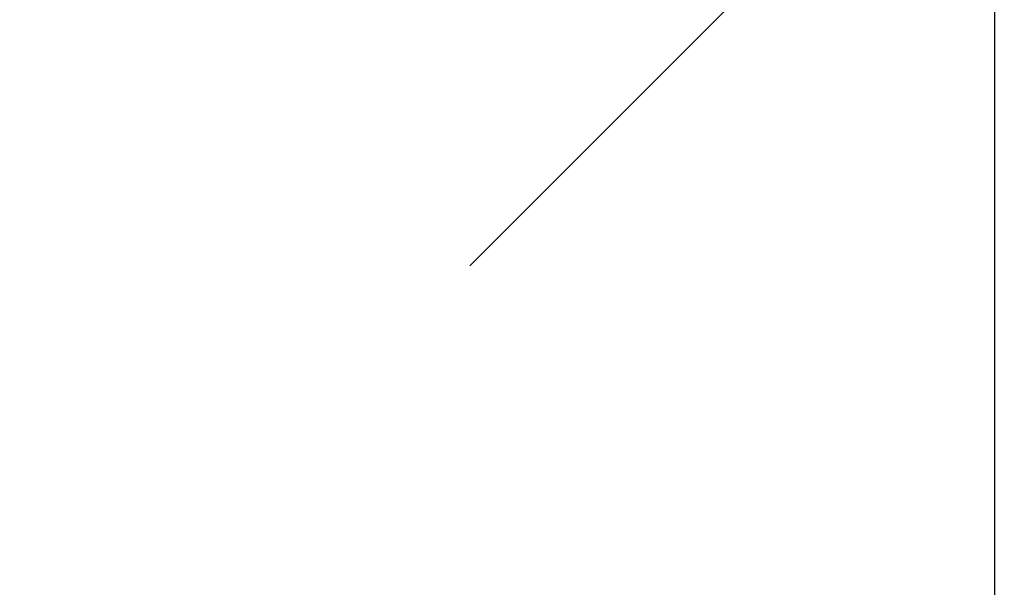
# Model space of a CAD drawing. Units: inches. Extents: x -1198 to -69, y -512 to 437.
# Tile 13 of 50: x -950.733 to -945.108, y 185.385 to 188.628. Entities that reach past the tile are written whole.
import ezdxf

# ---------------------------------------------------------------- set-up
doc = ezdxf.new("R2010")
doc.units = ezdxf.units.IN
doc.header["$MEASUREMENT"] = 0
doc.layers.add('A-ANNO-DIMS', color=2, linetype='Continuous', lineweight=18)
doc.styles.get("Standard").update_dxf_attribs({"font": 'arial.ttf'})
doc.dimstyles.get("Standard").update_dxf_attribs({"dimtxt": 6, "dimasz": 6, "dimexe": 0.18, "dimexo": 0.0625, "dimgap": 0.09, "dimtad": 0, "dimtih": 1, "dimtoh": 1, "dimdec": 0, "dimzin": 0, "dimdsep": 46, "dimlunit": 4, "dimtxsty": 'Standard', "dimblk": 'OBLIQUE', "dimcen": 0.09, "dimadec": 0, "dimazin": 0, "dimtfac": 1, "dimtdec": 0, "dimtofl": 0, "dimtmove": 0, "dimatfit": 3, "dimfxl": 1, "dimtolj": 1, "dimtzin": 0, "dimarcsym": 0})

# ---------------------------------------------------------------- blocks, each defined once
blk = doc.blocks.new('_Oblique')
at = {"color": 0, "linetype": 'ByBlock', "lineweight": -2}
blk.add_line((-0.5, -0.5), (0.5, 0.5), dxfattribs=at)
blk = doc.blocks.new('*D50')
at = {"layer": 'A-ANNO-DIMS', "color": 0, "lineweight": -2, "ltscale": 10, "transparency": 16777216}
for p, q in [((-978.4621, 185.2902), (-978.4621, 190.4026)), ((-945.1627, 185.2902), (-945.1627, 190.4026)), ((-978.4621, 190.2226), (-984.4621, 190.2226)), ((-945.1627, 190.2226), (-978.4621, 190.2226))]:
    blk.add_line(p, q, dxfattribs=at)
at = {"layer": 'DEFPOINTS', "color": 0, "ltscale": 10, "transparency": 16777216}
for p in [(-978.4621, 190.2226), (-978.4621, 185.2277), (-945.1627, 185.2277)]:
    blk.add_point(p, dxfattribs=at)
at = {"layer": 'A-ANNO-DIMS', "color": 0, "lineweight": -2, "ltscale": 10, "transparency": 16777216, "xscale": 6, "yscale": 6, "zscale": 6, "rotation": 180}
blk.add_blockref('_Oblique', (-978.4621, 190.2226), dxfattribs=at)
at = {"layer": 'A-ANNO-DIMS', "color": 0, "lineweight": -2, "ltscale": 10, "transparency": 16777216, "xscale": 6, "yscale": 6, "zscale": 6}
blk.add_blockref('_Oblique', (-945.1627, 190.2226), dxfattribs=at)
at = {"layer": 'A-ANNO-DIMS', "color": 0, "ltscale": 10, "transparency": 16777216, "insert": (-1009.2397, 190.2226), "char_height": 6, "attachment_point": 5}
blk.add_mtext('\\A1;HOB 33 TYP.', dxfattribs=at)

msp = doc.modelspace()

# ---------------------------------------------------------------- dimensions: what is measured, and where the dimension line sits
at = {"layer": 'A-ANNO-DIMS', "ltscale": 10}
dim = msp.add_linear_dim(base=(-978.4621, 190.2226), p1=(-945.1627, 185.2277), p2=(-978.4621, 185.2277), angle=180, text='HOB <> TYP.', dimstyle='Standard', override={"dimdec": 0, "dimlfac": 1, "dimrnd": 0, "dimzin": 0, "dimdsep": 46, "dimlunit": 2}, dxfattribs=at)
dim.commit()
dim.dimension.update_dxf_attribs({"geometry": '*D50', "text_midpoint": (-1009.2397, 190.2226)})

doc.saveas('drawing.dxf')
